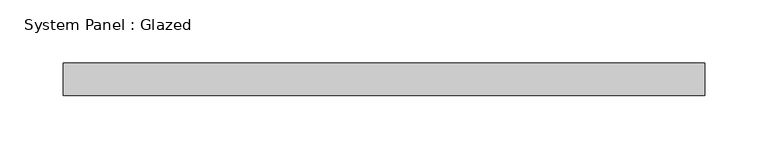
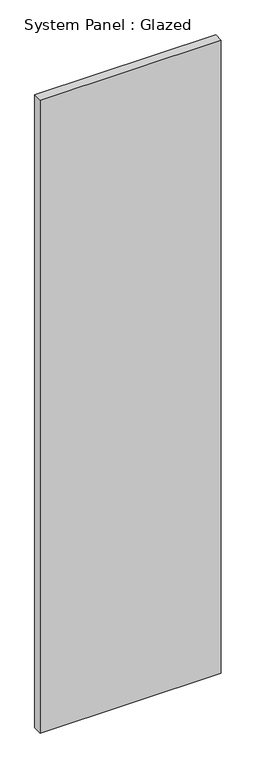
"""IFC4 building model written with IfcOpenShell, lengths in millimetres: plate geometry, System Panel : Glazed."""

from ifc_helpers import new_model, si_unit, origin, origin_with_axes, place, context, project, spatial, polyline, outline, extrude, source, transform, mapped, element, save


def system_panel_glazed_831ab98e(model_context):
    return source(origin(), model_context, "Body", "SweptSolid", [
        extrude(outline(polyline([(252.9416667, 19.05), (-252.9416667, 19.05), (-252.9416667, 44.45), (252.9416667, 44.45), (252.9416667, 19.05)])), origin_with_axes(), (0.0, 0.0, 1.0), 1868.867321),
    ])


if __name__ == "__main__":
    model = new_model("IFC4")
    model_context = context("Model", 3, world=origin())
    ifc_project = project(units=[si_unit("LENGTHUNIT", "METRE", prefix="MILLI")], contexts=[model_context])
    site = spatial("IfcSite", under=ifc_project)
    building = spatial("IfcBuilding", under=site)
    placement = place(None, origin())
    system_panel_glazed_shape = system_panel_glazed_831ab98e(model_context)
    element("IfcPlate", 1, ObjectType="System Panel : Glazed", at=placement, inside=building, context=model_context, shape_type="MappedRepresentation", body=[
        mapped(system_panel_glazed_shape, transform((0.0, 0.0, 0.0), x_axis=(1.0, 0.0, 0.0), y_axis=(0.0, 1.0, 0.0), z_axis=(0.0, 0.0, 1.0))),
    ])
    save(model, "model.ifc")

# Revit data of these elements
# Type "System Panel : Glazed"
#   Construction Type Id = "GSP4R"
#   Analytic Construction = "1/8 in Pilkington single glazing"
#   Visual Light Transmittance = 0.9
#   Solar Heat Gain Coefficient = 0.86
#   Heat Transfer Coefficient (U) = 1.18115 BTU/(h·ft²·°F)
#   Define Thermal Properties by = 1
# Element 1 (IfcPlate, "System Panel : Glazed")
#   Materials on its faces: "Glass"
# Materials
#   "Glass": class "Glass", colour RGB 0 128 192, transparency 0.75, Description = "Soda Lime Glass", Cost = 0
